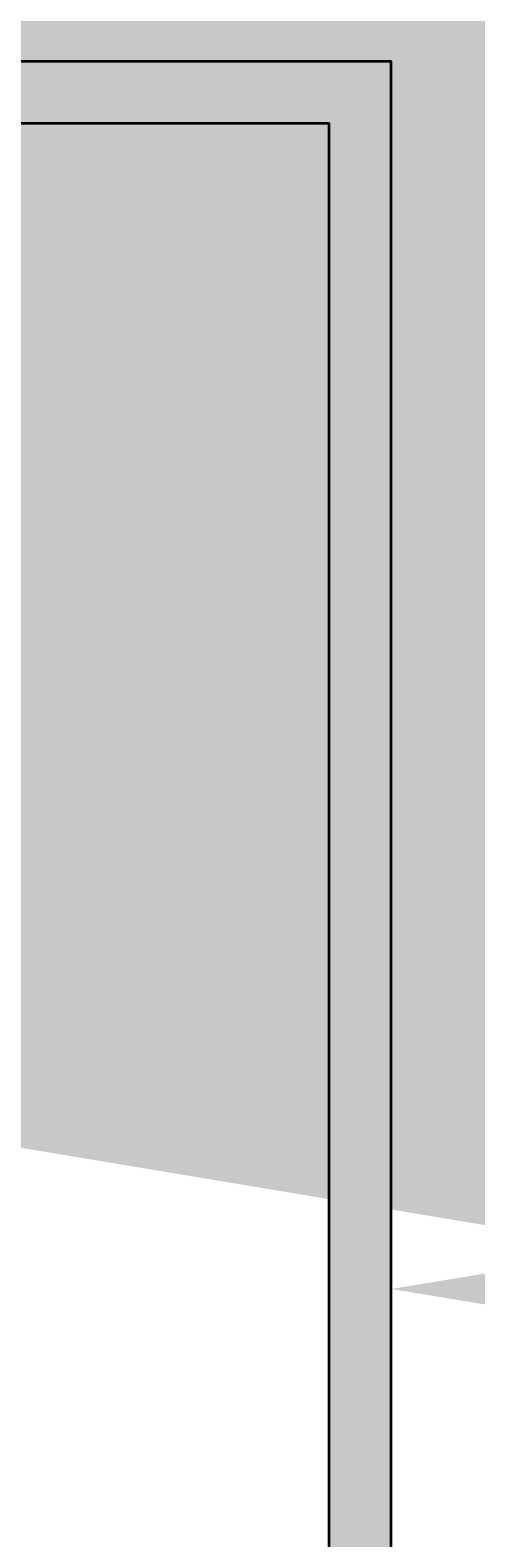
# Model space of a CAD drawing. Units: millimetres. Extents: x -22994 to 29398, y -19990 to 20176.
# Tile 41 of 135: x 183 to 190, y 54 to 78. Entities that reach past the tile are written whole.
import ezdxf
from ezdxf import colors
from ezdxf.entities.mleader import LeaderData, LeaderLine
from ezdxf.math import Vec2, Vec3

# ---------------------------------------------------------------- set-up
doc = ezdxf.new("R2010")
doc.units = ezdxf.units.MM
doc.header["$MEASUREMENT"] = 0
for name, color, linetype, lineweight in [('M-ANNO-TEXT', 7, 'Continuous', 25), ('M-DIMS', 2, 'Continuous', 18), ('M-EQPM-PATT', 7, 'Continuous', 18), ('M-PIPE', 7, 'Continuous', 35)]:
    doc.layers.add(name, color=color, linetype=linetype, lineweight=lineweight)
doc.styles.get("Standard").update_dxf_attribs({"font": 'arial.ttf'})
doc.dimstyles.get("Standard").update_dxf_attribs({"dimtxt": 0.18, "dimasz": 10000, "dimexe": 0.18, "dimexo": 0.0625, "dimgap": 0.09, "dimtad": 0, "dimtih": 1, "dimtoh": 1, "dimdec": 0, "dimzin": 0, "dimdsep": 46, "dimtxsty": 'Standard', "dimcen": 0.09, "dimadec": 0, "dimazin": 0, "dimtfac": 1, "dimtdec": 0, "dimtofl": 0, "dimtmove": 0, "dimatfit": 3, "dimfxl": 1, "dimtolj": 1, "dimtzin": 0, "dimlwd": 30, "dimarcsym": 0})

# ---------------------------------------------------------------- blocks, each defined once
blk = doc.blocks.new('*D2')
at = {"layer": 'Defpoints', "color": 0, "transparency": 16777216}
for p in [(6.677, 10.271), (290.852, 10.271), (290.852, -5.079)]:
    blk.add_point(p, dxfattribs=at)
at = {"layer": 'M-DIMS', "color": 0, "lineweight": -2, "transparency": 16777216}
for p, q in [((6.677, 10.209), (6.677, -5.259)), ((290.852, 10.209), (290.852, -5.259))]:
    blk.add_line(p, q, dxfattribs=at)
at = {"layer": 'M-DIMS', "color": 0, "lineweight": 30, "transparency": 16777216}
for p, q in [((-9993.323, -5.079), (-19993.323, -5.079)), ((10290.852, -5.079), (20290.852, -5.079))]:
    blk.add_line(p, q, dxfattribs=at)
at = {"layer": 'M-DIMS', "color": 0, "transparency": 16777216}
for points in [[(-9993.323, 1661.588), (-9993.323, -1671.745), (6.677, -5.079)], [(10290.852, 1661.588), (10290.852, -1671.745), (290.852, -5.079)]]:
    blk.add_solid(points, dxfattribs=at)
at = {"layer": 'M-DIMS', "color": 0, "transparency": 16777216, "insert": (148.765, -5.079), "char_height": 0.18, "attachment_point": 5}
blk.add_mtext('\\A1;284.2', dxfattribs=at)
blk = doc.blocks.new('*D3')
at = {"layer": 'Defpoints', "color": 0, "transparency": 16777216}
for p in [(110.265, 204.165), (110.265, 176.366), (95.833, 127.967)]:
    blk.add_point(p, dxfattribs=at)
at = {"layer": 'M-DIMS', "color": 0, "lineweight": -2, "transparency": 16777216}
for p, q in [((95.833, 128.03), (95.833, 204.345)), ((110.265, 176.429), (110.265, 204.345))]:
    blk.add_line(p, q, dxfattribs=at)
at = {"layer": 'M-DIMS', "color": 0, "lineweight": 30, "transparency": 16777216}
for p, q in [((-9904.167, 204.165), (-19904.167, 204.165)), ((10110.265, 204.165), (20110.265, 204.165))]:
    blk.add_line(p, q, dxfattribs=at)
at = {"layer": 'M-DIMS', "color": 0, "transparency": 16777216}
for points in [[(-9904.167, 1870.832), (-9904.167, -1462.501), (95.833, 204.165)], [(10110.265, 1870.832), (10110.265, -1462.501), (110.265, 204.165)]]:
    blk.add_solid(points, dxfattribs=at)
at = {"layer": 'M-DIMS', "color": 0, "transparency": 16777216, "insert": (103.049, 204.165), "char_height": 0.18, "attachment_point": 5}
blk.add_mtext('\\A1;14.432', dxfattribs=at)
blk = doc.blocks.new('*D4')
at = {"layer": 'Defpoints', "color": 0, "transparency": 16777216}
for p in [(116.265, 204.165), (110.265, 176.366), (116.265, 176.366)]:
    blk.add_point(p, dxfattribs=at)
at = {"layer": 'M-DIMS', "color": 0, "lineweight": -2, "transparency": 16777216}
for p, q in [((110.265, 176.429), (110.265, 204.345)), ((116.265, 176.429), (116.265, 204.345))]:
    blk.add_line(p, q, dxfattribs=at)
at = {"layer": 'M-DIMS', "color": 0, "lineweight": 30, "transparency": 16777216}
for p, q in [((-9889.735, 204.165), (-19889.735, 204.165)), ((10116.265, 204.165), (20116.265, 204.165))]:
    blk.add_line(p, q, dxfattribs=at)
at = {"layer": 'M-DIMS', "color": 0, "transparency": 16777216}
for points in [[(-9889.735, 1870.832), (-9889.735, -1462.501), (110.265, 204.165)], [(10116.265, 1870.832), (10116.265, -1462.501), (116.265, 204.165)]]:
    blk.add_solid(points, dxfattribs=at)
at = {"layer": 'M-DIMS', "color": 0, "transparency": 16777216, "insert": (113.265, 204.165), "char_height": 0.18, "attachment_point": 5}
blk.add_mtext('\\A1;6', dxfattribs=at)
blk = doc.blocks.new('*D5')
at = {"layer": 'Defpoints', "color": 0, "transparency": 16777216}
for p in [(181.265, 204.165), (116.265, 176.366), (181.265, 176.366)]:
    blk.add_point(p, dxfattribs=at)
at = {"layer": 'M-DIMS', "color": 0, "lineweight": -2, "transparency": 16777216}
for p, q in [((116.265, 176.429), (116.265, 204.345)), ((181.265, 176.429), (181.265, 204.345))]:
    blk.add_line(p, q, dxfattribs=at)
at = {"layer": 'M-DIMS', "color": 0, "lineweight": 30, "transparency": 16777216}
for p, q in [((-9883.735, 204.165), (-19883.735, 204.165)), ((10181.265, 204.165), (20181.265, 204.165))]:
    blk.add_line(p, q, dxfattribs=at)
at = {"layer": 'M-DIMS', "color": 0, "transparency": 16777216}
for points in [[(-9883.735, 1870.832), (-9883.735, -1462.501), (116.265, 204.165)], [(10181.265, 1870.832), (10181.265, -1462.501), (181.265, 204.165)]]:
    blk.add_solid(points, dxfattribs=at)
at = {"layer": 'M-DIMS', "color": 0, "transparency": 16777216, "insert": (148.765, 204.165), "char_height": 0.18, "attachment_point": 5}
blk.add_mtext('\\A1;65', dxfattribs=at)
blk = doc.blocks.new('*D6')
at = {"layer": 'Defpoints', "color": 0, "transparency": 16777216}
for p in [(187.265, 204.165), (181.265, 176.366), (187.265, 176.366)]:
    blk.add_point(p, dxfattribs=at)
at = {"layer": 'M-DIMS', "color": 0, "lineweight": -2, "transparency": 16777216}
for p, q in [((181.265, 176.429), (181.265, 204.345)), ((187.265, 176.429), (187.265, 204.345))]:
    blk.add_line(p, q, dxfattribs=at)
at = {"layer": 'M-DIMS', "color": 0, "lineweight": 30, "transparency": 16777216}
for p, q in [((-9818.735, 204.165), (-19818.735, 204.165)), ((10187.265, 204.165), (20187.265, 204.165))]:
    blk.add_line(p, q, dxfattribs=at)
at = {"layer": 'M-DIMS', "color": 0, "transparency": 16777216}
for points in [[(-9818.735, 1870.832), (-9818.735, -1462.501), (181.265, 204.165)], [(10187.265, 1870.832), (10187.265, -1462.501), (187.265, 204.165)]]:
    blk.add_solid(points, dxfattribs=at)
at = {"layer": 'M-DIMS', "color": 0, "transparency": 16777216, "insert": (184.265, 204.165), "char_height": 0.18, "attachment_point": 5}
blk.add_mtext('\\A1;6', dxfattribs=at)
blk = doc.blocks.new('*D7')
at = {"layer": 'Defpoints', "color": 0, "transparency": 16777216}
for p in [(201.697, 204.165), (187.265, 176.366), (201.697, 127.967)]:
    blk.add_point(p, dxfattribs=at)
at = {"layer": 'M-DIMS', "color": 0, "lineweight": -2, "transparency": 16777216}
for p, q in [((187.265, 176.429), (187.265, 204.345)), ((201.697, 128.03), (201.697, 204.345))]:
    blk.add_line(p, q, dxfattribs=at)
at = {"layer": 'M-DIMS', "color": 0, "lineweight": 30, "transparency": 16777216}
for p, q in [((-9812.735, 204.165), (-19812.735, 204.165)), ((10201.697, 204.165), (20201.697, 204.165))]:
    blk.add_line(p, q, dxfattribs=at)
at = {"layer": 'M-DIMS', "color": 0, "transparency": 16777216}
for points in [[(-9812.735, 1870.832), (-9812.735, -1462.501), (187.265, 204.165)], [(10201.697, 1870.832), (10201.697, -1462.501), (201.697, 204.165)]]:
    blk.add_solid(points, dxfattribs=at)
at = {"layer": 'M-DIMS', "color": 0, "transparency": 16777216, "insert": (194.481, 204.165), "char_height": 0.18, "attachment_point": 5}
blk.add_mtext('\\A1;14.432', dxfattribs=at)
blk = doc.blocks.new('*D8')
at = {"layer": 'Defpoints', "color": 0, "transparency": 16777216}
for p in [(227.648, 204.165), (227.648, 146.73), (201.697, 127.967)]:
    blk.add_point(p, dxfattribs=at)
at = {"layer": 'M-DIMS', "color": 0, "lineweight": -2, "transparency": 16777216}
for p, q in [((201.697, 128.03), (201.697, 204.345)), ((227.648, 146.792), (227.648, 204.345))]:
    blk.add_line(p, q, dxfattribs=at)
at = {"layer": 'M-DIMS', "color": 0, "lineweight": 30, "transparency": 16777216}
for p, q in [((-9798.303, 204.165), (-19798.303, 204.165)), ((10227.648, 204.165), (20227.648, 204.165))]:
    blk.add_line(p, q, dxfattribs=at)
at = {"layer": 'M-DIMS', "color": 0, "transparency": 16777216}
for points in [[(-9798.303, 1870.832), (-9798.303, -1462.501), (201.697, 204.165)], [(10227.648, 1870.832), (10227.648, -1462.501), (227.648, 204.165)]]:
    blk.add_solid(points, dxfattribs=at)
at = {"layer": 'M-DIMS', "color": 0, "transparency": 16777216, "insert": (214.673, 204.165), "char_height": 0.18, "attachment_point": 5}
blk.add_mtext('\\A1;25.95', dxfattribs=at)
blk = doc.blocks.new('*D9')
at = {"layer": 'Defpoints', "color": 0, "transparency": 16777216}
for p in [(187.265, 176.366), (306.202, 176.366), (290.852, 10.271)]:
    blk.add_point(p, dxfattribs=at)
at = {"layer": 'M-DIMS', "color": 0, "lineweight": 30, "transparency": 16777216}
for p, q in [((306.202, 10176.366), (306.202, 20176.366)), ((306.202, -9989.729), (306.202, -19989.729))]:
    blk.add_line(p, q, dxfattribs=at)
at = {"layer": 'M-DIMS', "color": 0, "lineweight": -2, "transparency": 16777216}
for p, q in [((187.327, 176.366), (306.382, 176.366)), ((290.915, 10.271), (306.382, 10.271))]:
    blk.add_line(p, q, dxfattribs=at)
at = {"layer": 'M-DIMS', "color": 0, "transparency": 16777216}
for points in [[(-1360.465, 10176.366), (1972.869, 10176.366), (306.202, 176.366)], [(-1360.465, -9989.729), (1972.869, -9989.729), (306.202, 10.271)]]:
    blk.add_solid(points, dxfattribs=at)
at = {"layer": 'M-DIMS', "color": 0, "transparency": 16777216, "insert": (306.202, 93.319), "char_height": 0.18, "attachment_point": 5}
blk.add_mtext('\\A1;166.1', dxfattribs=at)
blk = doc.blocks.new('*D10')
at = {"layer": 'Defpoints', "color": 0, "transparency": 16777216}
for p in [(125.65, 136.071), (133.346, 136.071), (133.346, -5.079)]:
    blk.add_point(p, dxfattribs=at)
at = {"layer": 'M-DIMS', "color": 0, "lineweight": -2, "transparency": 16777216}
for p, q in [((125.65, 136.009), (125.65, -5.259)), ((133.346, 136.009), (133.346, -5.259))]:
    blk.add_line(p, q, dxfattribs=at)
at = {"layer": 'M-DIMS', "color": 0, "lineweight": 30, "transparency": 16777216}
for p, q in [((-9874.35, -5.079), (-19874.35, -5.079)), ((10133.346, -5.079), (20133.346, -5.079))]:
    blk.add_line(p, q, dxfattribs=at)
at = {"layer": 'M-DIMS', "color": 0, "transparency": 16777216}
for points in [[(-9874.35, 1661.588), (-9874.35, -1671.745), (125.65, -5.079)], [(10133.346, 1661.588), (10133.346, -1671.745), (133.346, -5.079)]]:
    blk.add_solid(points, dxfattribs=at)
at = {"layer": 'M-DIMS', "color": 0, "transparency": 16777216, "insert": (129.498, -5.079), "char_height": 0.18, "attachment_point": 5}
blk.add_mtext('\\A1;7.696', dxfattribs=at)
blk = doc.blocks.new('*D11')
at = {"layer": 'Defpoints', "color": 0, "transparency": 16777216}
for p in [(133.346, 136.071), (135.65, 136.071), (135.65, -5.079)]:
    blk.add_point(p, dxfattribs=at)
at = {"layer": 'M-DIMS', "color": 0, "lineweight": -2, "transparency": 16777216}
for p, q in [((133.346, 136.009), (133.346, -5.259)), ((135.65, 136.009), (135.65, -5.259))]:
    blk.add_line(p, q, dxfattribs=at)
at = {"layer": 'M-DIMS', "color": 0, "lineweight": 30, "transparency": 16777216}
for p, q in [((-9866.654, -5.079), (-19866.654, -5.079)), ((10135.65, -5.079), (20135.65, -5.079))]:
    blk.add_line(p, q, dxfattribs=at)
at = {"layer": 'M-DIMS', "color": 0, "transparency": 16777216}
for points in [[(-9866.654, 1661.588), (-9866.654, -1671.745), (133.346, -5.079)], [(10135.65, 1661.588), (10135.65, -1671.745), (135.65, -5.079)]]:
    blk.add_solid(points, dxfattribs=at)
at = {"layer": 'M-DIMS', "color": 0, "transparency": 16777216, "insert": (134.498, -5.079), "char_height": 0.18, "attachment_point": 5}
blk.add_mtext('\\A1;2.304', dxfattribs=at)
blk = doc.blocks.new('*D12')
at = {"layer": 'Defpoints', "color": 0, "transparency": 16777216}
for p in [(135.65, 136.071), (145.65, 136.071), (145.65, -5.079)]:
    blk.add_point(p, dxfattribs=at)
at = {"layer": 'M-DIMS', "color": 0, "lineweight": -2, "transparency": 16777216}
for p, q in [((135.65, 136.009), (135.65, -5.259)), ((145.65, 136.009), (145.65, -5.259))]:
    blk.add_line(p, q, dxfattribs=at)
at = {"layer": 'M-DIMS', "color": 0, "lineweight": 30, "transparency": 16777216}
for p, q in [((-9864.35, -5.079), (-19864.35, -5.079)), ((10145.65, -5.079), (20145.65, -5.079))]:
    blk.add_line(p, q, dxfattribs=at)
at = {"layer": 'M-DIMS', "color": 0, "transparency": 16777216}
for points in [[(-9864.35, 1661.588), (-9864.35, -1671.745), (135.65, -5.079)], [(10145.65, 1661.588), (10145.65, -1671.745), (145.65, -5.079)]]:
    blk.add_solid(points, dxfattribs=at)
at = {"layer": 'M-DIMS', "color": 0, "transparency": 16777216, "insert": (140.65, -5.079), "char_height": 0.18, "attachment_point": 5}
blk.add_mtext('\\A1;10', dxfattribs=at)
blk = doc.blocks.new('*D13')
at = {"layer": 'Defpoints', "color": 0, "transparency": 16777216}
for p in [(145.65, 136.071), (155.65, 136.071), (155.65, -5.079)]:
    blk.add_point(p, dxfattribs=at)
at = {"layer": 'M-DIMS', "color": 0, "lineweight": -2, "transparency": 16777216}
for p, q in [((145.65, 136.009), (145.65, -5.259)), ((155.65, 136.009), (155.65, -5.259))]:
    blk.add_line(p, q, dxfattribs=at)
at = {"layer": 'M-DIMS', "color": 0, "lineweight": 30, "transparency": 16777216}
for p, q in [((-9854.35, -5.079), (-19854.35, -5.079)), ((10155.65, -5.079), (20155.65, -5.079))]:
    blk.add_line(p, q, dxfattribs=at)
at = {"layer": 'M-DIMS', "color": 0, "transparency": 16777216}
for points in [[(-9854.35, 1661.588), (-9854.35, -1671.745), (145.65, -5.079)], [(10155.65, 1661.588), (10155.65, -1671.745), (155.65, -5.079)]]:
    blk.add_solid(points, dxfattribs=at)
at = {"layer": 'M-DIMS', "color": 0, "transparency": 16777216, "insert": (150.65, -5.079), "char_height": 0.18, "attachment_point": 5}
blk.add_mtext('\\A1;10', dxfattribs=at)
blk = doc.blocks.new('*D14')
at = {"layer": 'Defpoints', "color": 0, "transparency": 16777216}
for p in [(155.65, 136.071), (165.65, 136.071), (165.65, -5.079)]:
    blk.add_point(p, dxfattribs=at)
at = {"layer": 'M-DIMS', "color": 0, "lineweight": -2, "transparency": 16777216}
for p, q in [((155.65, 136.009), (155.65, -5.259)), ((165.65, 136.009), (165.65, -5.259))]:
    blk.add_line(p, q, dxfattribs=at)
at = {"layer": 'M-DIMS', "color": 0, "lineweight": 30, "transparency": 16777216}
for p, q in [((-9844.35, -5.079), (-19844.35, -5.079)), ((10165.65, -5.079), (20165.65, -5.079))]:
    blk.add_line(p, q, dxfattribs=at)
at = {"layer": 'M-DIMS', "color": 0, "transparency": 16777216}
for points in [[(-9844.35, 1661.588), (-9844.35, -1671.745), (155.65, -5.079)], [(10165.65, 1661.588), (10165.65, -1671.745), (165.65, -5.079)]]:
    blk.add_solid(points, dxfattribs=at)
at = {"layer": 'M-DIMS', "color": 0, "transparency": 16777216, "insert": (160.65, -5.079), "char_height": 0.18, "attachment_point": 5}
blk.add_mtext('\\A1;10', dxfattribs=at)
blk = doc.blocks.new('*D15')
at = {"layer": 'Defpoints', "color": 0, "transparency": 16777216}
for p in [(173.346, 154.788), (173.346, 136.071), (306.202, 136.071)]:
    blk.add_point(p, dxfattribs=at)
at = {"layer": 'M-DIMS', "color": 0, "lineweight": 30, "transparency": 16777216}
for p, q in [((306.202, 10154.788), (306.202, 20154.788)), ((306.202, -9863.929), (306.202, -19863.929))]:
    blk.add_line(p, q, dxfattribs=at)
at = {"layer": 'M-DIMS', "color": 0, "lineweight": -2, "transparency": 16777216}
for p, q in [((173.408, 154.788), (306.382, 154.788)), ((173.408, 136.071), (306.382, 136.071))]:
    blk.add_line(p, q, dxfattribs=at)
at = {"layer": 'M-DIMS', "color": 0, "transparency": 16777216}
for points in [[(-1360.465, 10154.788), (1972.869, 10154.788), (306.202, 154.788)], [(-1360.465, -9863.929), (1972.869, -9863.929), (306.202, 136.071)]]:
    blk.add_solid(points, dxfattribs=at)
at = {"layer": 'M-DIMS', "color": 0, "transparency": 16777216, "insert": (306.202, 145.43), "char_height": 0.18, "attachment_point": 5}
blk.add_mtext('\\A1;18.717', dxfattribs=at)
blk = doc.blocks.new('*D16')
at = {"layer": 'Defpoints', "color": 0, "transparency": 16777216}
for p in [(120.17, 204.165), (110.466, 48.035), (120.17, 48.035)]:
    blk.add_point(p, dxfattribs=at)
at = {"layer": 'M-DIMS', "color": 0, "lineweight": -2, "transparency": 16777216}
for p, q in [((110.466, 48.097), (110.466, 204.345)), ((120.17, 48.097), (120.17, 204.345))]:
    blk.add_line(p, q, dxfattribs=at)
at = {"layer": 'M-DIMS', "color": 0, "lineweight": 30, "transparency": 16777216}
for p, q in [((-9889.534, 204.165), (-19889.534, 204.165)), ((10120.17, 204.165), (20120.17, 204.165))]:
    blk.add_line(p, q, dxfattribs=at)
at = {"layer": 'M-DIMS', "color": 0, "transparency": 16777216}
for points in [[(-9889.534, 1870.832), (-9889.534, -1462.501), (110.466, 204.165)], [(10120.17, 1870.832), (10120.17, -1462.501), (120.17, 204.165)]]:
    blk.add_solid(points, dxfattribs=at)
at = {"layer": 'M-DIMS', "color": 0, "transparency": 16777216, "insert": (115.318, 204.165), "char_height": 0.18, "attachment_point": 5}
blk.add_mtext('\\A1;9.704', dxfattribs=at)
blk = doc.blocks.new('*D17')
at = {"layer": 'Defpoints', "color": 0, "transparency": 16777216}
for p in [(126.17, 204.165), (120.17, 48.035), (126.17, 48.035)]:
    blk.add_point(p, dxfattribs=at)
at = {"layer": 'M-DIMS', "color": 0, "lineweight": -2, "transparency": 16777216}
for p, q in [((120.17, 48.097), (120.17, 204.345)), ((126.17, 48.097), (126.17, 204.345))]:
    blk.add_line(p, q, dxfattribs=at)
at = {"layer": 'M-DIMS', "color": 0, "lineweight": 30, "transparency": 16777216}
for p, q in [((-9879.83, 204.165), (-19879.83, 204.165)), ((10126.17, 204.165), (20126.17, 204.165))]:
    blk.add_line(p, q, dxfattribs=at)
at = {"layer": 'M-DIMS', "color": 0, "transparency": 16777216}
for points in [[(-9879.83, 1870.832), (-9879.83, -1462.501), (120.17, 204.165)], [(10126.17, 1870.832), (10126.17, -1462.501), (126.17, 204.165)]]:
    blk.add_solid(points, dxfattribs=at)
at = {"layer": 'M-DIMS', "color": 0, "transparency": 16777216, "insert": (123.17, 204.165), "char_height": 0.18, "attachment_point": 5}
blk.add_mtext('\\A1;6', dxfattribs=at)
blk = doc.blocks.new('*D18')
at = {"layer": 'Defpoints', "color": 0, "transparency": 16777216}
for p in [(132.17, 204.165), (126.17, 48.035), (132.17, 48.035)]:
    blk.add_point(p, dxfattribs=at)
at = {"layer": 'M-DIMS', "color": 0, "lineweight": -2, "transparency": 16777216}
for p, q in [((126.17, 48.097), (126.17, 204.345)), ((132.17, 48.097), (132.17, 204.345))]:
    blk.add_line(p, q, dxfattribs=at)
at = {"layer": 'M-DIMS', "color": 0, "lineweight": 30, "transparency": 16777216}
for p, q in [((-9873.83, 204.165), (-19873.83, 204.165)), ((10132.17, 204.165), (20132.17, 204.165))]:
    blk.add_line(p, q, dxfattribs=at)
at = {"layer": 'M-DIMS', "color": 0, "transparency": 16777216}
for points in [[(-9873.83, 1870.832), (-9873.83, -1462.501), (126.17, 204.165)], [(10132.17, 1870.832), (10132.17, -1462.501), (132.17, 204.165)]]:
    blk.add_solid(points, dxfattribs=at)
at = {"layer": 'M-DIMS', "color": 0, "transparency": 16777216, "insert": (129.17, 204.165), "char_height": 0.18, "attachment_point": 5}
blk.add_mtext('\\A1;6', dxfattribs=at)
blk = doc.blocks.new('*D19')
at = {"layer": 'Defpoints', "color": 0, "transparency": 16777216}
for p in [(138.17, 204.165), (132.17, 48.035), (138.17, 48.035)]:
    blk.add_point(p, dxfattribs=at)
at = {"layer": 'M-DIMS', "color": 0, "lineweight": -2, "transparency": 16777216}
for p, q in [((132.17, 48.097), (132.17, 204.345)), ((138.17, 48.097), (138.17, 204.345))]:
    blk.add_line(p, q, dxfattribs=at)
at = {"layer": 'M-DIMS', "color": 0, "lineweight": 30, "transparency": 16777216}
for p, q in [((-9867.83, 204.165), (-19867.83, 204.165)), ((10138.17, 204.165), (20138.17, 204.165))]:
    blk.add_line(p, q, dxfattribs=at)
at = {"layer": 'M-DIMS', "color": 0, "transparency": 16777216}
for points in [[(-9867.83, 1870.832), (-9867.83, -1462.501), (132.17, 204.165)], [(10138.17, 1870.832), (10138.17, -1462.501), (138.17, 204.165)]]:
    blk.add_solid(points, dxfattribs=at)
at = {"layer": 'M-DIMS', "color": 0, "transparency": 16777216, "insert": (135.17, 204.165), "char_height": 0.18, "attachment_point": 5}
blk.add_mtext('\\A1;6', dxfattribs=at)
blk = doc.blocks.new('*D20')
at = {"layer": 'Defpoints', "color": 0, "transparency": 16777216}
for p in [(144.17, 204.165), (138.17, 48.035), (144.17, 48.035)]:
    blk.add_point(p, dxfattribs=at)
at = {"layer": 'M-DIMS', "color": 0, "lineweight": -2, "transparency": 16777216}
for p, q in [((138.17, 48.097), (138.17, 204.345)), ((144.17, 48.097), (144.17, 204.345))]:
    blk.add_line(p, q, dxfattribs=at)
at = {"layer": 'M-DIMS', "color": 0, "lineweight": 30, "transparency": 16777216}
for p, q in [((-9861.83, 204.165), (-19861.83, 204.165)), ((10144.17, 204.165), (20144.17, 204.165))]:
    blk.add_line(p, q, dxfattribs=at)
at = {"layer": 'M-DIMS', "color": 0, "transparency": 16777216}
for points in [[(-9861.83, 1870.832), (-9861.83, -1462.501), (138.17, 204.165)], [(10144.17, 1870.832), (10144.17, -1462.501), (144.17, 204.165)]]:
    blk.add_solid(points, dxfattribs=at)
at = {"layer": 'M-DIMS', "color": 0, "transparency": 16777216, "insert": (141.17, 204.165), "char_height": 0.18, "attachment_point": 5}
blk.add_mtext('\\A1;6', dxfattribs=at)
blk = doc.blocks.new('*D21')
at = {"layer": 'Defpoints', "color": 0, "transparency": 16777216}
for p in [(149.116, 204.165), (144.17, 48.035), (149.116, 48.035)]:
    blk.add_point(p, dxfattribs=at)
at = {"layer": 'M-DIMS', "color": 0, "lineweight": -2, "transparency": 16777216}
for p, q in [((144.17, 48.097), (144.17, 204.345)), ((149.116, 48.097), (149.116, 204.345))]:
    blk.add_line(p, q, dxfattribs=at)
at = {"layer": 'M-DIMS', "color": 0, "lineweight": 30, "transparency": 16777216}
for p, q in [((-9855.83, 204.165), (-19855.83, 204.165)), ((10149.116, 204.165), (20149.116, 204.165))]:
    blk.add_line(p, q, dxfattribs=at)
at = {"layer": 'M-DIMS', "color": 0, "transparency": 16777216}
for points in [[(-9855.83, 1870.832), (-9855.83, -1462.501), (144.17, 204.165)], [(10149.116, 1870.832), (10149.116, -1462.501), (149.116, 204.165)]]:
    blk.add_solid(points, dxfattribs=at)
at = {"layer": 'M-DIMS', "color": 0, "transparency": 16777216, "insert": (146.643, 204.165), "char_height": 0.18, "attachment_point": 5}
blk.add_mtext('\\A1;4.945', dxfattribs=at)
blk = doc.blocks.new('*D22')
at = {"layer": 'Defpoints', "color": 0, "transparency": 16777216}
for p in [(149.116, 30.99), (155.116, 30.99), (155.116, -5.079)]:
    blk.add_point(p, dxfattribs=at)
at = {"layer": 'M-DIMS', "color": 0, "lineweight": -2, "transparency": 16777216}
for p, q in [((149.116, 30.927), (149.116, -5.259)), ((155.116, 30.927), (155.116, -5.259))]:
    blk.add_line(p, q, dxfattribs=at)
at = {"layer": 'M-DIMS', "color": 0, "lineweight": 30, "transparency": 16777216}
for p, q in [((-9850.884, -5.079), (-19850.884, -5.079)), ((10155.116, -5.079), (20155.116, -5.079))]:
    blk.add_line(p, q, dxfattribs=at)
at = {"layer": 'M-DIMS', "color": 0, "transparency": 16777216}
for points in [[(-9850.884, 1661.588), (-9850.884, -1671.745), (149.116, -5.079)], [(10155.116, 1661.588), (10155.116, -1671.745), (155.116, -5.079)]]:
    blk.add_solid(points, dxfattribs=at)
at = {"layer": 'M-DIMS', "color": 0, "transparency": 16777216, "insert": (152.116, -5.079), "char_height": 0.18, "attachment_point": 5}
blk.add_mtext('\\A1;6', dxfattribs=at)
blk = doc.blocks.new('*D23')
at = {"layer": 'Defpoints', "color": 0, "transparency": 16777216}
for p in [(155.116, 30.99), (161.116, 30.99), (161.116, -5.079)]:
    blk.add_point(p, dxfattribs=at)
at = {"layer": 'M-DIMS', "color": 0, "lineweight": -2, "transparency": 16777216}
for p, q in [((155.116, 30.927), (155.116, -5.259)), ((161.116, 30.927), (161.116, -5.259))]:
    blk.add_line(p, q, dxfattribs=at)
at = {"layer": 'M-DIMS', "color": 0, "lineweight": 30, "transparency": 16777216}
for p, q in [((-9844.884, -5.079), (-19844.884, -5.079)), ((10161.116, -5.079), (20161.116, -5.079))]:
    blk.add_line(p, q, dxfattribs=at)
at = {"layer": 'M-DIMS', "color": 0, "transparency": 16777216}
for points in [[(-9844.884, 1661.588), (-9844.884, -1671.745), (155.116, -5.079)], [(10161.116, 1661.588), (10161.116, -1671.745), (161.116, -5.079)]]:
    blk.add_solid(points, dxfattribs=at)
at = {"layer": 'M-DIMS', "color": 0, "transparency": 16777216, "insert": (158.116, -5.079), "char_height": 0.18, "attachment_point": 5}
blk.add_mtext('\\A1;6', dxfattribs=at)
blk = doc.blocks.new('*D24')
at = {"layer": 'Defpoints', "color": 0, "transparency": 16777216}
for p in [(161.116, 30.99), (166.439, 30.99), (166.439, -5.079)]:
    blk.add_point(p, dxfattribs=at)
at = {"layer": 'M-DIMS', "color": 0, "lineweight": -2, "transparency": 16777216}
for p, q in [((161.116, 30.927), (161.116, -5.259)), ((166.439, 30.927), (166.439, -5.259))]:
    blk.add_line(p, q, dxfattribs=at)
at = {"layer": 'M-DIMS', "color": 0, "lineweight": 30, "transparency": 16777216}
for p, q in [((-9838.884, -5.079), (-19838.884, -5.079)), ((10166.439, -5.079), (20166.439, -5.079))]:
    blk.add_line(p, q, dxfattribs=at)
at = {"layer": 'M-DIMS', "color": 0, "transparency": 16777216}
for points in [[(-9838.884, 1661.588), (-9838.884, -1671.745), (161.116, -5.079)], [(10166.439, 1661.588), (10166.439, -1671.745), (166.439, -5.079)]]:
    blk.add_solid(points, dxfattribs=at)
at = {"layer": 'M-DIMS', "color": 0, "transparency": 16777216, "insert": (163.777, -5.079), "char_height": 0.18, "attachment_point": 5}
blk.add_mtext('\\A1;5.323', dxfattribs=at)
blk = doc.blocks.new('*D25')
at = {"layer": 'Defpoints', "color": 0, "transparency": 16777216}
for p in [(166.439, 30.99), (172.439, 30.99), (172.439, -5.079)]:
    blk.add_point(p, dxfattribs=at)
at = {"layer": 'M-DIMS', "color": 0, "lineweight": -2, "transparency": 16777216}
for p, q in [((166.439, 30.927), (166.439, -5.259)), ((172.439, 30.927), (172.439, -5.259))]:
    blk.add_line(p, q, dxfattribs=at)
at = {"layer": 'M-DIMS', "color": 0, "lineweight": 30, "transparency": 16777216}
for p, q in [((-9833.561, -5.079), (-19833.561, -5.079)), ((10172.439, -5.079), (20172.439, -5.079))]:
    blk.add_line(p, q, dxfattribs=at)
at = {"layer": 'M-DIMS', "color": 0, "transparency": 16777216}
for points in [[(-9833.561, 1661.588), (-9833.561, -1671.745), (166.439, -5.079)], [(10172.439, 1661.588), (10172.439, -1671.745), (172.439, -5.079)]]:
    blk.add_solid(points, dxfattribs=at)
at = {"layer": 'M-DIMS', "color": 0, "transparency": 16777216, "insert": (169.439, -5.079), "char_height": 0.18, "attachment_point": 5}
blk.add_mtext('\\A1;6', dxfattribs=at)
blk = doc.blocks.new('*D26')
at = {"layer": 'Defpoints', "color": 0, "transparency": 16777216}
for p in [(172.439, 30.99), (178.439, 30.99), (178.439, -5.079)]:
    blk.add_point(p, dxfattribs=at)
at = {"layer": 'M-DIMS', "color": 0, "lineweight": -2, "transparency": 16777216}
for p, q in [((172.439, 30.927), (172.439, -5.259)), ((178.439, 30.927), (178.439, -5.259))]:
    blk.add_line(p, q, dxfattribs=at)
at = {"layer": 'M-DIMS', "color": 0, "lineweight": 30, "transparency": 16777216}
for p, q in [((-9827.561, -5.079), (-19827.561, -5.079)), ((10178.439, -5.079), (20178.439, -5.079))]:
    blk.add_line(p, q, dxfattribs=at)
at = {"layer": 'M-DIMS', "color": 0, "transparency": 16777216}
for points in [[(-9827.561, 1661.588), (-9827.561, -1671.745), (172.439, -5.079)], [(10178.439, 1661.588), (10178.439, -1671.745), (178.439, -5.079)]]:
    blk.add_solid(points, dxfattribs=at)
at = {"layer": 'M-DIMS', "color": 0, "transparency": 16777216, "insert": (175.439, -5.079), "char_height": 0.18, "attachment_point": 5}
blk.add_mtext('\\A1;6', dxfattribs=at)
blk = doc.blocks.new('*D27')
at = {"layer": 'Defpoints', "color": 0, "transparency": 16777216}
for p in [(178.439, 30.99), (188.117, 30.99), (188.117, -5.079)]:
    blk.add_point(p, dxfattribs=at)
at = {"layer": 'M-DIMS', "color": 0, "lineweight": -2, "transparency": 16777216}
for p, q in [((178.439, 30.927), (178.439, -5.259)), ((188.117, 30.927), (188.117, -5.259))]:
    blk.add_line(p, q, dxfattribs=at)
at = {"layer": 'M-DIMS', "color": 0, "lineweight": 30, "transparency": 16777216}
for p, q in [((-9821.561, -5.079), (-19821.561, -5.079)), ((10188.117, -5.079), (20188.117, -5.079))]:
    blk.add_line(p, q, dxfattribs=at)
at = {"layer": 'M-DIMS', "color": 0, "transparency": 16777216}
for points in [[(-9821.561, 1661.588), (-9821.561, -1671.745), (178.439, -5.079)], [(10188.117, 1661.588), (10188.117, -1671.745), (188.117, -5.079)]]:
    blk.add_solid(points, dxfattribs=at)
at = {"layer": 'M-DIMS', "color": 0, "transparency": 16777216, "insert": (183.278, -5.079), "char_height": 0.18, "attachment_point": 5}
blk.add_mtext('\\A1;9.679', dxfattribs=at)
blk = doc.blocks.new('*D28')
at = {"layer": 'Defpoints', "color": 0, "transparency": 16777216}
for p in [(188.117, 48.035), (306.202, 48.035), (188.117, 30.99)]:
    blk.add_point(p, dxfattribs=at)
at = {"layer": 'M-DIMS', "color": 0, "lineweight": 30, "transparency": 16777216}
for p, q in [((306.202, 10048.035), (306.202, 20048.035)), ((306.202, -9969.01), (306.202, -19969.01))]:
    blk.add_line(p, q, dxfattribs=at)
at = {"layer": 'M-DIMS', "color": 0, "lineweight": -2, "transparency": 16777216}
for p, q in [((188.18, 48.035), (306.382, 48.035)), ((188.18, 30.99), (306.382, 30.99))]:
    blk.add_line(p, q, dxfattribs=at)
at = {"layer": 'M-DIMS', "color": 0, "transparency": 16777216}
for points in [[(-1360.465, 10048.035), (1972.869, 10048.035), (306.202, 48.035)], [(-1360.465, -9969.01), (1972.869, -9969.01), (306.202, 30.99)]]:
    blk.add_solid(points, dxfattribs=at)
at = {"layer": 'M-DIMS', "color": 0, "transparency": 16777216, "insert": (306.202, 39.512), "char_height": 0.18, "attachment_point": 5}
blk.add_mtext('\\A1;17.045', dxfattribs=at)
blk = doc.blocks.new('*D29')
at = {"layer": 'Defpoints', "color": 0, "transparency": 16777216}
for p in [(36.801, 80.045), (64.03, 80.045)]:
    blk.add_point(p, dxfattribs=at)
at = {"layer": 'M-DIMS', "color": 0, "lineweight": -2, "transparency": 16777216}
for p, q in [((50.325, 80.045), (50.505, 80.045)), ((50.415, 79.955), (50.415, 80.135))]:
    blk.add_line(p, q, dxfattribs=at)
at = {"layer": 'M-DIMS', "color": 0, "lineweight": 30, "transparency": 16777216}
blk.add_line((20064.03, 80.03), (10064.03, 80.038), dxfattribs=at)
at = {"layer": 'M-DIMS', "color": 0, "transparency": 16777216}
blk.add_solid([(10064.031, 1746.704), (10064.028, -1586.629), (64.03, 80.045)], dxfattribs=at)
at = {"layer": 'M-DIMS', "color": 0, "transparency": 16777216, "insert": (20064.521, 80.03), "char_height": 0.18, "attachment_point": 5}
blk.add_mtext('\\A1;∅27.23', dxfattribs=at)
blk = doc.blocks.new('*D36')
at = {"layer": 'Defpoints', "color": 0, "transparency": 16777216}
for p in [(46.39, 31.303), (46.387, 26.593)]:
    blk.add_point(p, dxfattribs=at)
at = {"layer": 'M-DIMS', "color": 0, "lineweight": 30, "transparency": 16777216}
for p, q in [((57.15, 20031.301), (51.77, 10031.302)), ((10057.15, 20031.301), (57.15, 20031.301))]:
    blk.add_line(p, q, dxfattribs=at)
at = {"layer": 'M-DIMS', "color": 0, "lineweight": -2, "transparency": 16777216}
for p, q in [((46.299, 28.948), (46.479, 28.948)), ((46.389, 28.858), (46.389, 29.038))]:
    blk.add_line(p, q, dxfattribs=at)
at = {"layer": 'M-DIMS', "color": 0, "transparency": 16777216}
blk.add_solid([(-1614.896, 10032.199), (1718.436, 10030.405), (46.39, 31.303)], dxfattribs=at)
at = {"layer": 'M-DIMS', "color": 0, "transparency": 16777216, "insert": (10057.554, 20031.301), "char_height": 0.18, "attachment_point": 5}
blk.add_mtext('\\A1;∅4.71', dxfattribs=at)
blk = doc.blocks.new('*D37')
at = {"layer": 'Defpoints', "color": 0, "transparency": 16777216}
for p in [(54.834, 118.615), (59.494, 118.614)]:
    blk.add_point(p, dxfattribs=at)
at = {"layer": 'M-DIMS', "color": 0, "lineweight": -2, "transparency": 16777216}
for p, q in [((57.074, 118.614), (57.254, 118.614)), ((57.164, 118.524), (57.164, 118.704))]:
    blk.add_line(p, q, dxfattribs=at)
at = {"layer": 'M-DIMS', "color": 0, "lineweight": 30, "transparency": 16777216}
blk.add_line((20059.493, 116.253), (10059.494, 117.434), dxfattribs=at)
at = {"layer": 'M-DIMS', "color": 0, "transparency": 16777216}
blk.add_solid([(10059.69, 1784.1), (10059.297, -1549.233), (59.494, 118.614)], dxfattribs=at)
at = {"layer": 'M-DIMS', "color": 0, "transparency": 16777216, "insert": (20059.985, 116.253), "char_height": 0.18, "attachment_point": 5}
blk.add_mtext('\\A1;∅4.659', dxfattribs=at)

msp = doc.modelspace()

# ---------------------------------------------------------------- hatches: boundary and pattern name
at = {"layer": 'M-EQPM-PATT'}
h = msp.add_hatch(color=256, dxfattribs=at)
h.set_gradient(color1=(19, 155, 72), color2=(88, 186, 72), tint=1, name='CYLINDER')
h.paths.add_polyline_path([(109.4658, 29.9895), (189.1175, 29.9895), (189.1175, 77.6953), (128.1172, 77.6953, 0.4142136), (126.1172, 75.6953), (126.1172, 73.6953, 0.4142136), (128.1172, 71.6953), (178.5136, 71.6953, -0.4142136), (179.5136, 70.6953), (179.5136, 68.6953, -0.4142136), (178.5136, 67.6953), (128.1172, 67.6953, 0.4142136), (126.1172, 65.6953), (126.1172, 63.6953, 0.4142136), (128.1172, 61.6953), (178.5136, 61.6953, -0.4142136), (179.5136, 60.6953), (179.5136, 58.6953, -0.4142136), (178.5136, 57.6953), (109.7466, 57.6953, -0.4142136), (108.7466, 58.6953), (108.7466, 75.5922, 0.4142136), (106.7466, 77.5922), (101.8327, 77.5922), (101.8327, 76.5922), (106.7466, 76.5922, -0.4142136), (107.7466, 75.5922), (107.7466, 58.6953, 0.4142136), (109.7466, 56.6953), (178.5136, 56.6953, 0.4142136), (180.5136, 58.6953), (180.5136, 60.6953, 0.4142136), (178.5136, 62.6953), (128.1172, 62.6953, -0.4142136), (127.1172, 63.6953), (127.1172, 65.6953, -0.4142136), (128.1172, 66.6953), (178.5136, 66.6953, 0.4142136), (180.5136, 68.6953), (180.5136, 70.6953, 0.4142136), (178.5136, 72.6953), (128.1172, 72.6953, -0.4142136), (127.1172, 73.6953), (127.1172, 75.6953, -0.4142136), (128.1172, 76.6953), (188.1175, 76.6953), (188.1175, 49.0349), (110.4658, 49.0349), (110.4658, 51.9576), (101.8327, 51.9576), (101.8327, 50.9576), (109.4658, 50.9576), (109.4658, 48.5349)])
h.paths.add_polyline_path([(110.4658, 48.0349), (188.1175, 48.0349), (188.1175, 30.9895), (110.4658, 30.9895)], flags=16)
h.paths.add_polyline_path([(136.1519, 78.0082), (161.2406, 78.0082), (161.2406, 84.1903), (136.1519, 84.1903)], flags=9)

# ---------------------------------------------------------------- linework, layer by layer
at = {"layer": 'M-PIPE'}
for points in [[(189.1175, 29.9895), (189.1175, 77.6953), (128.1172, 77.6953, 0.4142136), (126.1172, 75.6953), (126.1172, 73.6953, 0.4142136), (128.1172, 71.6953), (178.5136, 71.6953, -0.4142136), (179.5136, 70.6953), (179.5136, 68.6953, -0.4142136), (178.5136, 67.6953), (128.1172, 67.6953, 0.4142136), (126.1172, 65.6953), (126.1172, 63.6953, 0.4142136), (128.1172, 61.6953), (178.5136, 61.6953, -0.4142136), (179.5136, 60.6953), (179.5136, 58.6953, -0.4142136), (178.5136, 57.6953), (109.7466, 57.6953, -0.4142136), (108.7466, 58.6953), (108.7466, 75.5922, 0.4142136), (106.7466, 77.5922), (101.8327, 77.5922)], [(188.1175, 49.0349), (188.1175, 76.6953), (128.1172, 76.6953, 0.4142136), (127.1172, 75.6953), (127.1172, 73.6953, 0.4142136), (128.1172, 72.6953), (178.5136, 72.6953, -0.4142136), (180.5136, 70.6953), (180.5136, 68.6953, -0.4142136), (178.5136, 66.6953), (128.1172, 66.6953, 0.4142136), (127.1172, 65.6953), (127.1172, 63.6953, 0.4142136), (128.1172, 62.6953), (178.5136, 62.6953, -0.4142136), (180.5136, 60.6953), (180.5136, 58.6953, -0.4142136), (178.5136, 56.6953), (109.7466, 56.6953, -0.4142136), (107.7466, 58.6953), (107.7466, 75.5922, 0.4142136), (106.7466, 76.5922), (101.8327, 76.5922)]]:
    msp.add_lwpolyline(points, format="xyb", dxfattribs=at)

# ---------------------------------------------------------------- dimensions: what is measured, and where the dimension line sits
at = {"layer": 'M-DIMS'}
for base, p1, p2, override, picture, middle in [((306.202, 176.3662), (290.852, 10.2713), (187.2647, 176.3662), {"dimdec": 1, "dimlfac": 1, "dimrnd": 0, "dimzin": 0, "dimdsep": 46, "dimlunit": 2}, '*D9', (306.202, 93.3187)), ((306.202, 136.0713), (173.3459, 154.788), (173.3459, 136.0713), {"dimdec": 3, "dimlfac": 1, "dimrnd": 0, "dimzin": 0, "dimdsep": 46, "dimlunit": 2}, '*D15', (306.202, 145.4297)), ((306.202, 48.0349), (188.1175, 30.9895), (188.1175, 48.0349), {"dimdec": 3, "dimlfac": 1, "dimrnd": 0, "dimzin": 0, "dimdsep": 46, "dimlunit": 2}, '*D28', (306.202, 39.5122))]:
    dim = msp.add_linear_dim(base=base, p1=p1, p2=p2, angle=90, dimstyle='Standard', override=override, dxfattribs=at)
    dim.commit()
    dim.dimension.update_dxf_attribs({"geometry": picture, "text_midpoint": middle})
dim = msp.add_diameter_dim_2p(p1=(46.3875, 26.5934), p2=(46.39, 31.3035), dimstyle='Standard', override={"dimdec": 2, "dimlfac": 1, "dimrnd": 0, "dimzin": 0, "dimdsep": 46, "dimlunit": 2}, dxfattribs=at)
dim.commit()
dim.dimension.update_dxf_attribs({"geometry": '*D36', "text_midpoint": (10057.5542, 20031.3006), "dimtype": 163})
for base, p1, p2, override, picture, middle in [((110.2647, 204.1654), (95.8327, 127.967), (110.2647, 176.3662), {"dimdec": 3, "dimlfac": 1, "dimrnd": 0, "dimzin": 0, "dimdsep": 46, "dimlunit": 2}, '*D3', (103.0487, 204.1654)), ((116.2647, 204.1654), (110.2647, 176.3662), (116.2647, 176.3662), {"dimdec": 0, "dimlfac": 1, "dimrnd": 0, "dimzin": 0, "dimdsep": 46, "dimlunit": 2}, '*D4', (113.2647, 204.1654)), ((120.1702, 204.1654), (110.4658, 48.0349), (120.1702, 48.0349), {"dimdec": 3, "dimlfac": 1, "dimrnd": 0, "dimzin": 0, "dimdsep": 46, "dimlunit": 2}, '*D16', (115.318, 204.1654)), ((181.2647, 204.1654), (116.2647, 176.3662), (181.2647, 176.3662), {"dimdec": 0, "dimlfac": 1, "dimrnd": 0, "dimzin": 0, "dimdsep": 46, "dimlunit": 2}, '*D5', (148.7647, 204.1654)), ((126.1702, 204.1654), (120.1702, 48.0349), (126.1702, 48.0349), {"dimdec": 0, "dimlfac": 1, "dimrnd": 0, "dimzin": 0, "dimdsep": 46, "dimlunit": 2}, '*D17', (123.1702, 204.1654)), ((132.1702, 204.1654), (126.1702, 48.0349), (132.1702, 48.0349), {"dimdec": 0, "dimlfac": 1, "dimrnd": 0, "dimzin": 0, "dimdsep": 46, "dimlunit": 2}, '*D18', (129.1702, 204.1654)), ((138.1702, 204.1654), (132.1702, 48.0349), (138.1702, 48.0349), {"dimdec": 0, "dimlfac": 1, "dimrnd": 0, "dimzin": 0, "dimdsep": 46, "dimlunit": 2}, '*D19', (135.1702, 204.1654)), ((144.1702, 204.1654), (138.1702, 48.0349), (144.1702, 48.0349), {"dimdec": 0, "dimlfac": 1, "dimrnd": 0, "dimzin": 0, "dimdsep": 46, "dimlunit": 2}, '*D20', (141.1702, 204.1654)), ((149.11567, 204.16539), (144.17023, 48.03494), (149.11567, 48.03494), {"dimdec": 3, "dimlfac": 1, "dimrnd": 0, "dimzin": 0, "dimdsep": 46, "dimlunit": 2}, '*D21', (146.64295, 204.16539)), ((187.2647, 204.1654), (181.2647, 176.3662), (187.2647, 176.3662), {"dimdec": 0, "dimlfac": 1, "dimrnd": 0, "dimzin": 0, "dimdsep": 46, "dimlunit": 2}, '*D6', (184.2647, 204.1654)), ((201.6967, 204.1654), (187.2647, 176.3662), (201.6967, 127.967), {"dimdec": 3, "dimlfac": 1, "dimrnd": 0, "dimzin": 0, "dimdsep": 46, "dimlunit": 2}, '*D7', (194.4807, 204.1654)), ((227.6485, 204.1654), (201.6967, 127.967), (227.6485, 146.7296), {"dimdec": 2, "dimlfac": 1, "dimrnd": 0, "dimzin": 0, "dimdsep": 46, "dimlunit": 2}, '*D8', (214.6726, 204.1654)), ((290.852, -5.0787), (6.6773, 10.2713), (290.852, 10.2713), {"dimdec": 1, "dimlfac": 1, "dimrnd": 0, "dimzin": 0, "dimdsep": 46, "dimlunit": 2}, '*D2', (148.7647, -5.0787)), ((133.3459, -5.0787), (125.6498, 136.0713), (133.3459, 136.0713), {"dimdec": 3, "dimlfac": 1, "dimrnd": 0, "dimzin": 0, "dimdsep": 46, "dimlunit": 2}, '*D10', (129.4978, -5.0787)), ((135.6498, -5.0787), (133.3459, 136.0713), (135.6498, 136.0713), {"dimdec": 3, "dimlfac": 1, "dimrnd": 0, "dimzin": 0, "dimdsep": 46, "dimlunit": 2}, '*D11', (134.4978, -5.0787)), ((145.6498, -5.0787), (135.6498, 136.0713), (145.6498, 136.0713), {"dimdec": 0, "dimlfac": 1, "dimrnd": 0, "dimzin": 0, "dimdsep": 46, "dimlunit": 2}, '*D12', (140.6498, -5.0787)), ((155.6498, -5.0787), (145.6498, 136.0713), (155.6498, 136.0713), {"dimdec": 0, "dimlfac": 1, "dimrnd": 0, "dimzin": 0, "dimdsep": 46, "dimlunit": 2}, '*D13', (150.6498, -5.0787)), ((155.1157, -5.0787), (149.1157, 30.9895), (155.1157, 30.9895), {"dimdec": 0, "dimlfac": 1, "dimrnd": 0, "dimzin": 0, "dimdsep": 46, "dimlunit": 2}, '*D22', (152.1157, -5.0787)), ((161.1157, -5.0787), (155.1157, 30.9895), (161.1157, 30.9895), {"dimdec": 0, "dimlfac": 1, "dimrnd": 0, "dimzin": 0, "dimdsep": 46, "dimlunit": 2}, '*D23', (158.1157, -5.0787)), ((165.6498, -5.0787), (155.6498, 136.0713), (165.6498, 136.0713), {"dimdec": 0, "dimlfac": 1, "dimrnd": 0, "dimzin": 0, "dimdsep": 46, "dimlunit": 2}, '*D14', (160.6498, -5.0787)), ((166.4387, -5.0787), (161.1157, 30.9895), (166.4387, 30.9895), {"dimdec": 3, "dimlfac": 1, "dimrnd": 0, "dimzin": 0, "dimdsep": 46, "dimlunit": 2}, '*D24', (163.7772, -5.0787)), ((172.4387, -5.0787), (166.4387, 30.9895), (172.4387, 30.9895), {"dimdec": 0, "dimlfac": 1, "dimrnd": 0, "dimzin": 0, "dimdsep": 46, "dimlunit": 2}, '*D25', (169.4387, -5.0787)), ((178.4387, -5.0787), (172.4387, 30.9895), (178.4387, 30.9895), {"dimdec": 0, "dimlfac": 1, "dimrnd": 0, "dimzin": 0, "dimdsep": 46, "dimlunit": 2}, '*D26', (175.4387, -5.0787)), ((188.1175, -5.0787), (178.4387, 30.9895), (188.1175, 30.9895), {"dimdec": 3, "dimlfac": 1, "dimrnd": 0, "dimzin": 0, "dimdsep": 46, "dimlunit": 2}, '*D27', (183.2781, -5.0787))]:
    dim = msp.add_linear_dim(base=base, p1=p1, p2=p2, dimstyle='Standard', override=override, dxfattribs=at)
    dim.commit()
    dim.dimension.update_dxf_attribs({"geometry": picture, "text_midpoint": middle})
for p1, p2, override, picture, middle in [((54.8343, 118.6145), (59.4936, 118.614), {"dimdec": 3, "dimlfac": 1, "dimrnd": 0, "dimzin": 0, "dimdsep": 46, "dimlunit": 2}, '*D37', (20059.4934, 116.2531)), ((36.8006, 80.045), (64.0296, 80.045), {"dimdec": 2, "dimlfac": 1, "dimrnd": 0, "dimzin": 0, "dimdsep": 46, "dimlunit": 2}, '*D29', (20064.0296, 80.0303))]:
    dim = msp.add_diameter_dim_2p(p1=p1, p2=p2, dimstyle='Standard', override=override, dxfattribs=at)
    dim.commit()
    dim.dimension.update_dxf_attribs({"geometry": picture, "text_midpoint": middle})

# ---------------------------------------------------------------- leaders
at = {"layer": 'M-ANNO-TEXT'}
ml = msp.add_multileader_mtext('Standard', dxfattribs=at)
ml.set_content('combustion chamber', color=256)
ml.set_leader_properties()
ml.build(insert=Vec2(0, 0))
ml.multileader.update_dxf_attribs({"dogleg_length": 0.36, "arrow_head_size": 200})
ctx = ml.context
ctx.base_point, ctx.char_height, ctx.arrow_head_size, ctx.landing_gap_size, ctx.plane_origin = Vec3(215.7321, 57.9149), 3, 200, 0.09, Vec3(189.1175, 57.9149)
notes = []
notes.append((ctx, [(0, (1, 1, 0), (215.3721, 57.9149), (1, 0), 0.36, [(0, [(189.1175, 57.9149)], 0, [])])]))
ctx.mtext.insert, ctx.mtext.flow_direction = Vec3(215.8221, 59.4394), 5
for ctx, leaders in notes:
    for number, flags, end, landing, length, lines in leaders:
        leader = LeaderData()
        leader.index, (leader.has_last_leader_line, leader.has_dogleg_vector, leader.attachment_direction) = number, flags
        leader.last_leader_point, leader.dogleg_vector, leader.dogleg_length = Vec3(end), Vec3(landing), length
        for number, points, colour, breaks in lines:
            line = LeaderLine()
            line.index, line.vertices, line.color, line.breaks = number, Vec3.list(points), colors.encode_raw_color(colour), breaks
            leader.lines.append(line)
        ctx.leaders.append(leader)

doc.saveas('drawing.dxf')
